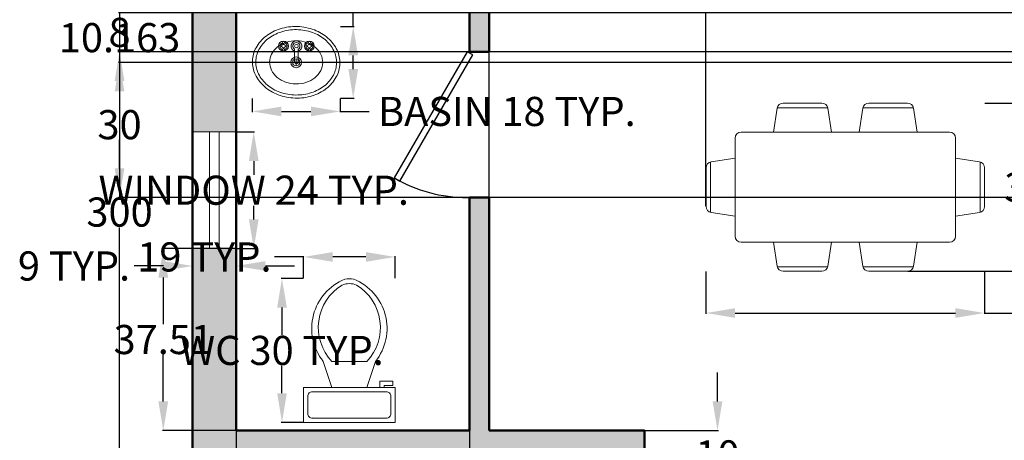
# Model space of a CAD drawing. Units: inches. Extents: x -11 to 341, y -300 to 41.
# Tile 2 of 5: x -11 to 192, y -178 to -91. Entities that reach past the tile are written whole.
import ezdxf

# ---------------------------------------------------------------- set-up
doc = ezdxf.new("R2010")
doc.units = ezdxf.units.IN
doc.header["$MEASUREMENT"] = 0
for name, color, linetype, lineweight in [('A-ANNO-DIMS', 2, 'Continuous', 18), ('A-DOOR', 3, 'Continuous', 25), ('A-FLOR-FIXT', 9, 'Continuous', 18), ('A-FURN', 8, 'Continuous', 18), ('A-GLAZ', 4, 'Continuous', 18), ('A-WALL', 7, 'Continuous', 50), ('A-WALL-PATT', 251, 'Continuous', 13)]:
    doc.layers.add(name, color=color, linetype=linetype, lineweight=lineweight)
doc.styles.get("Standard").update_dxf_attribs({"font": 'arial.ttf'})
doc.dimstyles.get("Standard").update_dxf_attribs({"dimtxt": 6, "dimasz": 6, "dimexe": 0.18, "dimexo": 0.0625, "dimgap": 0.09, "dimtad": 0, "dimtih": 1, "dimtoh": 1, "dimdec": 0, "dimzin": 0, "dimdsep": 46, "dimlunit": 4, "dimtxsty": 'Standard', "dimcen": 0.09, "dimadec": 0, "dimazin": 0, "dimtfac": 1, "dimtdec": 0, "dimtofl": 0, "dimtmove": 0, "dimatfit": 3, "dimfxl": 1, "dimtolj": 1, "dimtzin": 0, "dimarcsym": 0})

# ---------------------------------------------------------------- blocks, each defined once
blk = doc.blocks.new('*U15')
for p, q in [((0, 0), (0, 6)), ((40, 0), (40, 6))]:
    blk.add_line(p, q)
blk.add_lwpolyline([(0, 0), (34.64, -20), (35.52, -18.48), (0.87, 1.52)], close=True)
blk.add_arc((0, 0), 40, 330, 0)
blk = doc.blocks.new('Toilet - top')
for p, q in [((9.5, -6), (9.5, -2)), ((-10, -8.5), (-8, -8.5)), ((-10, -9.5), (-10, -8.5)), ((-8, -8.5), (-8, -8)), ((-7, -8), (-7, -9.5)), ((-4, -8), (-6, -14)), ((4, -8), (6, -14)), ((-7, -9.5), (-10, -9.5)), ((4, -14), (-4, -14))]:
    blk.add_line(p, q)
blk.add_lwpolyline([(10.5, -8), (10.5, 0), (-10.5, 0), (-10.5, -8)], close=True)
for points in [[(-9.5, -2), (-9.5, -6)], [(8.5, -1), (-8.5, -1)], [(-8.5, -7), (8.5, -7)]]:
    blk.add_lwpolyline(points)
for centre, radius, start, end in [((-8.62, -1.88), 0.884, 81.8699, 188.1301), ((8.62, -1.88), 0.884, 351.8699, 98.1301), ((-8.62, -6.12), 0.884, 171.8699, 278.1301), ((8.62, -6.12), 0.884, 261.8699, 8.1301), ((3.52, -21.58), 12.17, 141.4691, 247.9714), ((4.2, -21.82), 11.33, 136.3677, 238.9468), ((-3.52, -21.58), 12.17, 292.0284, 38.5307), ((-4.2, -21.82), 11.33, 301.053, 43.6321), ((0, -27.88), 4, 245.7318, 294.2682), ((0, -29), 4, 254.8605, 285.1395)]:
    blk.add_arc(centre, radius, start, end)
blk = doc.blocks.new('Sink - Oval top')
for p, q in [((-1, 0), (1, 0)), ((0, 1), (0, -1))]:
    blk.add_line(p, q)
for points in [[(-12.23, 0.39, 0.117634), (-11.46, -3.36, 0.104469), (-8.88, -6.8, 0.090016), (-5.08, -9.07, 0.08192), (-0.32, -10.02, 0.08192), (4.49, -9.38, 0.090016), (8.42, -7.36, 0.104469), (11.22, -4.09, 0.117634), (12.23, -0.39, 0.117634), (11.46, 3.36, 0.104469), (8.88, 6.8, 0.090016), (5.08, 9.07, 0.08192), (0.32, 10.02, 0.08192), (-4.49, 9.38, 0.090016), (-8.42, 7.36, 0.104469), (-11.22, 4.09, 0.117634)], [(-11.29, 0.16, 0.118622), (-10.52, -3.25, 0.104678), (-8.07, -6.36, 0.089562), (-4.54, -8.37, 0.081185), (-0.13, -9.15, 0.081185), (4.3, -8.49, 0.089562), (7.89, -6.58, 0.104678), (10.42, -3.55, 0.118622), (11.29, -0.16, 0.118622), (10.52, 3.25, 0.104678), (8.07, 6.36, 0.089562), (4.54, 8.37, 0.081185), (0.13, 9.15, 0.081185), (-4.3, 8.49, 0.089562), (-7.89, 6.58, 0.104678), (-10.42, 3.55, 0.118622)], [(-7.42, 0.08, 0.118283), (-6.91, -2.17, 0.104607), (-5.29, -4.21, 0.089718), (-2.97, -5.53, 0.081436), (-0.07, -6.04, 0.081436), (2.84, -5.59, 0.089718), (5.2, -4.33, 0.104607), (6.86, -2.32, 0.118283), (7.42, -0.08, 0.118283), (6.91, 2.17, 0.104607), (5.29, 4.21, 0.089718), (2.97, 5.53, 0.081436), (0.07, 6.04, 0.081436), (-2.84, 5.59, 0.089718), (-5.2, 4.33, 0.104607), (-6.86, 2.32, 0.118283)]]:
    blk.add_lwpolyline(points, format="xyb", close=True)
for radius in [1.5, 1]:
    blk.add_circle((0, 0), radius)
blk = doc.blocks.new('Faucet - Bathroom top')
for p, q in [((-4.107, 0.125), (-4.375, 0.125)), ((-3.75, 0.4788), (-3.75, 0.75)), ((-3.5, 0.482), (-3.5, 0.75)), ((-3.1461, 0.125), (-2.875, 0.125)), ((3.143, 0.125), (2.875, 0.125)), ((3.5, 0.4788), (3.5, 0.75)), ((3.75, 0.482), (3.75, 0.75)), ((4.1039, 0.125), (4.375, 0.125)), ((-4.1039, -0.125), (-4.375, -0.125)), ((-3.75, -0.4821), (-3.75, -0.75)), ((-3.5, -0.4789), (-3.5, -0.75)), ((-3.143, -0.125), (-2.875, -0.125)), ((-0.5, -0.8639), (-0.5, -4.5)), ((0.5, -4.5), (0.5, -0.8631)), ((3.1461, -0.125), (2.875, -0.125)), ((3.5, -0.4821), (3.5, -0.75)), ((3.75, -0.4789), (3.75, -0.75)), ((4.107, -0.125), (4.375, -0.125))]:
    blk.add_line(p, q)
for centre, radius in [((-3.625, 0), 1.375), ((-4.625, 0), 0.2795), ((-3.625, 0), 0.5), ((-3.625, 1), 0.2795), ((-2.625, 0), 0.2795), ((0, 0), 0.5), ((3.625, 0), 1.375), ((2.625, 0), 0.2795), ((3.625, 0), 0.5), ((3.625, 1), 0.2795), ((4.625, 0), 0.2795), ((-3.625, -1), 0.2795), ((3.625, -1), 0.2795)]:
    blk.add_circle(centre, radius)
for centre, radius, start, end in [((-3.625, 0), 1, 105.2407, 164.2093), ((-3.625, 0), 1, 16.44125, 74.07887), ((0, 0), 1.5, 289.6514, 250.3603), ((0, 0), 1, 300.3431, 239.7554), ((3.625, 0), 1, 106.12, 164.0884), ((3.625, 0), 1, 16.23422, 73.90469), ((-3.625, 0), 1, 196.2342, 253.9047), ((-3.625, 0), 1, 286.12, 344.0884), ((3.625, 0), 1, 196.4413, 254.0789), ((3.625, 0), 1, 285.2407, 344.2093), ((0, -4.5), 0.5, 180, 0)]:
    blk.add_arc(centre, radius, start, end)
blk = doc.blocks.new('Dining Set - 36 x 72 in.')
for p, q in [((-22.26, 25.81), (-23.48, 18)), ((-22.23, 26), (-5.76, 26)), ((-20.29, 27.5), (-7.71, 27.5)), ((-4.52, 18), (-5.74, 25.81)), ((5.74, 25.81), (4.52, 18)), ((5.77, 26), (22.24, 26)), ((7.71, 27.5), (20.29, 27.5)), ((23.48, 18), (22.26, 25.81)), ((34, 18), (-34, 18)), ((-36, 16), (-36, -16)), ((36, -16), (36, 16)), ((-44, 8.23), (-44, -8.24)), ((-43.81, 8.26), (-36, 9.48)), ((43.81, 8.26), (36, 9.48)), ((44, 8.23), (44, -8.24)), ((-45.5, 6.29), (-45.5, -6.29)), ((45.5, 6.29), (45.5, -6.29)), ((-36, -9.48), (-43.81, -8.26)), ((36, -9.48), (43.81, -8.26)), ((-34, -18), (34, -18)), ((-22.26, -25.81), (-23.48, -18)), ((-4.52, -18), (-5.74, -25.81)), ((5.74, -25.81), (4.52, -18)), ((23.48, -18), (22.26, -25.81)), ((-22.23, -26), (-5.76, -26)), ((-20.29, -27.5), (-7.71, -27.5)), ((5.77, -26), (22.24, -26)), ((7.71, -27.5), (20.29, -27.5))]:
    blk.add_line(p, q)
for centre, start, end in [((-20.29, 25.5), 90, 171.1198), ((-7.71, 25.5), 8.881, 90), ((7.71, 25.5), 90, 171.1198), ((20.29, 25.5), 8.881, 90), ((-34, 16), 90, 180), ((34, 16), 0, 90), ((-43.5, 6.29), 98.8806, 180), ((43.5, 6.29), 0, 81.1194), ((-43.5, -6.29), 180, 261.1194), ((43.5, -6.29), 278.8806, 0), ((-34, -16), 180, 270), ((34, -16), 270, 0), ((-20.29, -25.5), 188.8802, 270), ((-7.71, -25.5), 270, 351.1191), ((7.71, -25.5), 188.8802, 270), ((20.29, -25.5), 270, 351.1191)]:
    blk.add_arc(centre, 2, start, end)
blk = doc.blocks.new('WIN-24IN')
for p, q in [((0, 24), (9, 24)), ((3.5, 0), (3.5, 24)), ((5.5, 0), (5.5, 24)), ((9, 0), (0, 0))]:
    blk.add_line(p, q)
blk = doc.blocks.new('*D21')
at = {"layer": 'A-ANNO-DIMS', "color": 0, "lineweight": -2, "transparency": 16777216}
for p, q in [((33.63, -114.1), (37.35, -114.1)), ((37.17, -120.1), (37.17, -122.9)), ((37.17, -132.1), (37.17, -129.29)), ((33.63, -138.1), (37.35, -138.1))]:
    blk.add_line(p, q, dxfattribs=at)
at = {"layer": 'A-ANNO-DIMS', "color": 0, "transparency": 16777216}
for points in [[(36.17, -120.1), (38.17, -120.1), (37.17, -114.1)], [(36.17, -132.1), (38.17, -132.1), (37.17, -138.1)]]:
    blk.add_solid(points, dxfattribs=at)
at = {"layer": 'Defpoints', "color": 0, "transparency": 16777216}
for p in [(33.57, -114.1), (33.57, -138.1), (37.17, -138.1)]:
    blk.add_point(p, dxfattribs=at)
at = {"layer": 'A-ANNO-DIMS', "color": 0, "transparency": 16777216, "insert": (37.17, -126.1), "char_height": 6, "attachment_point": 5}
blk.add_mtext('\\A1;WINDOW 24 TYP.', dxfattribs=at)
blk = doc.blocks.new('*D22')
at = {"layer": 'A-ANNO-DIMS', "color": 0, "lineweight": -2, "transparency": 16777216}
for p, q in [((24.57, -138.16), (24.57, -141.88)), ((33.57, -138.16), (33.57, -141.88)), ((18.57, -141.7), (12.57, -141.7)), ((39.57, -141.7), (45.57, -141.7))]:
    blk.add_line(p, q, dxfattribs=at)
at = {"layer": 'A-ANNO-DIMS', "color": 0, "transparency": 16777216}
for points in [[(18.57, -140.7), (18.57, -142.7), (24.57, -141.7)], [(39.57, -140.7), (39.57, -142.7), (33.57, -141.7)]]:
    blk.add_solid(points, dxfattribs=at)
at = {"layer": 'Defpoints', "color": 0, "transparency": 16777216}
for p in [(24.57, -138.1), (33.57, -138.1), (24.57, -141.7)]:
    blk.add_point(p, dxfattribs=at)
at = {"layer": 'A-ANNO-DIMS', "color": 0, "transparency": 16777216, "insert": (0.2, -141.7), "char_height": 6, "attachment_point": 5}
blk.add_mtext('\\A1;9 TYP.', dxfattribs=at)
blk = doc.blocks.new('*D29')
at = {"layer": 'A-ANNO-DIMS', "color": 0, "lineweight": -2, "transparency": 16777216}
for p, q in [((47.36, -144.28), (42.8, -144.28)), ((42.98, -150.28), (42.98, -155.9)), ((42.98, -167.9), (42.98, -162.29)), ((47.36, -173.9), (42.8, -173.9))]:
    blk.add_line(p, q, dxfattribs=at)
at = {"layer": 'A-ANNO-DIMS', "color": 0, "transparency": 16777216}
for points in [[(41.98, -150.28), (43.98, -150.28), (42.98, -144.28)], [(41.98, -167.9), (43.98, -167.9), (42.98, -173.9)]]:
    blk.add_solid(points, dxfattribs=at)
at = {"layer": 'Defpoints', "color": 0, "transparency": 16777216}
for p in [(47.43, -144.28), (42.98, -173.9), (47.43, -173.9)]:
    blk.add_point(p, dxfattribs=at)
at = {"layer": 'A-ANNO-DIMS', "color": 0, "transparency": 16777216, "insert": (42.98, -159.09), "char_height": 6, "attachment_point": 5}
blk.add_mtext('\\A1;WC 30 TYP.', dxfattribs=at)
blk = doc.blocks.new('*D30')
at = {"layer": 'A-ANNO-DIMS', "color": 0, "lineweight": -2, "transparency": 16777216}
for p, q in [((47.43, -144.22), (47.43, -139.66)), ((66.25, -144.22), (66.25, -139.66)), ((47.43, -139.84), (41.43, -139.84)), ((60.25, -139.84), (53.43, -139.84))]:
    blk.add_line(p, q, dxfattribs=at)
at = {"layer": 'A-ANNO-DIMS', "color": 0, "transparency": 16777216}
for points in [[(53.43, -138.84), (53.43, -140.84), (47.43, -139.84)], [(60.25, -138.84), (60.25, -140.84), (66.25, -139.84)]]:
    blk.add_solid(points, dxfattribs=at)
at = {"layer": 'Defpoints', "color": 0, "transparency": 16777216}
for p in [(47.43, -139.84), (47.43, -144.28), (66.25, -144.28)]:
    blk.add_point(p, dxfattribs=at)
at = {"layer": 'A-ANNO-DIMS', "color": 0, "transparency": 16777216, "insert": (27.02, -139.84), "char_height": 6, "attachment_point": 5}
blk.add_mtext('\\A1;19 TYP.', dxfattribs=at)
blk = doc.blocks.new('*D31')
at = {"layer": 'A-ANNO-DIMS', "color": 0, "lineweight": -2, "transparency": 16777216}
for p, q in [((36.87, -107.23), (36.87, -110.06)), ((54.93, -107.23), (54.93, -110.06)), ((42.87, -109.88), (48.93, -109.88)), ((54.93, -109.88), (60.93, -109.88))]:
    blk.add_line(p, q, dxfattribs=at)
at = {"layer": 'A-ANNO-DIMS', "color": 0, "transparency": 16777216}
for points in [[(42.87, -108.88), (42.87, -110.88), (36.87, -109.88)], [(48.93, -108.88), (48.93, -110.88), (54.93, -109.88)]]:
    blk.add_solid(points, dxfattribs=at)
at = {"layer": 'Defpoints', "color": 0, "transparency": 16777216}
for p in [(36.87, -107.17), (54.93, -107.17), (54.93, -109.88)]:
    blk.add_point(p, dxfattribs=at)
at = {"layer": 'A-ANNO-DIMS', "color": 0, "transparency": 16777216, "insert": (89.23, -109.88), "char_height": 6, "attachment_point": 5}
blk.add_mtext('\\A1;BASIN 18 TYP.', dxfattribs=at)
blk = doc.blocks.new('*D32')
at = {"layer": 'A-ANNO-DIMS', "color": 0, "lineweight": -2, "transparency": 16777216}
for p, q in [((57.63, -92.36), (57.63, -86.36)), ((57.63, -86.36), (63.63, -86.36)), ((54.99, -92.36), (57.81, -92.36)), ((57.63, -101.17), (57.63, -98.36)), ((54.99, -107.17), (57.81, -107.17))]:
    blk.add_line(p, q, dxfattribs=at)
at = {"layer": 'A-ANNO-DIMS', "color": 0, "transparency": 16777216}
for points in [[(56.63, -98.36), (58.63, -98.36), (57.63, -92.36)], [(56.63, -101.17), (58.63, -101.17), (57.63, -107.17)]]:
    blk.add_solid(points, dxfattribs=at)
at = {"layer": 'Defpoints', "color": 0, "transparency": 16777216}
for p in [(54.93, -92.36), (57.63, -92.36), (54.93, -107.17)]:
    blk.add_point(p, dxfattribs=at)
at = {"layer": 'A-ANNO-DIMS', "color": 0, "transparency": 16777216, "insert": (78.05, -86.36), "char_height": 6, "attachment_point": 5}
blk.add_mtext('\\A1;15 TYP.', dxfattribs=at)
blk = doc.blocks.new('*D43')
at = {"layer": 'A-ANNO-DIMS', "color": 0, "lineweight": -2, "transparency": 16777216}
for p, q in [((130.2, -142.86), (130.2, -151.57)), ((187.51, -142.86), (187.51, -151.57)), ((136.2, -151.39), (181.51, -151.39)), ((187.51, -151.39), (193.51, -151.39))]:
    blk.add_line(p, q, dxfattribs=at)
at = {"layer": 'A-ANNO-DIMS', "color": 0, "transparency": 16777216}
for points in [[(136.2, -150.39), (136.2, -152.39), (130.2, -151.39)], [(181.51, -150.39), (181.51, -152.39), (187.51, -151.39)]]:
    blk.add_solid(points, dxfattribs=at)
at = {"layer": 'Defpoints', "color": 0, "transparency": 16777216}
for p in [(130.2, -142.8), (187.51, -142.8), (187.51, -151.39)]:
    blk.add_point(p, dxfattribs=at)
at = {"layer": 'A-ANNO-DIMS', "color": 0, "transparency": 16777216, "insert": (222.9, -151.39), "char_height": 6, "attachment_point": 5}
blk.add_mtext('\\A1;DINING SET 57', dxfattribs=at)
blk = doc.blocks.new('*D44')
at = {"layer": 'A-ANNO-DIMS', "color": 0, "lineweight": -2, "transparency": 16777216}
for p, q in [((187.57, -108.16), (196.29, -108.16)), ((196.11, -114.16), (196.11, -122.32)), ((196.11, -136.8), (196.11, -128.63)), ((187.57, -142.8), (196.29, -142.8))]:
    blk.add_line(p, q, dxfattribs=at)
at = {"layer": 'A-ANNO-DIMS', "color": 0, "transparency": 16777216}
for points in [[(195.11, -114.16), (197.11, -114.16), (196.11, -108.16)], [(195.11, -136.8), (197.11, -136.8), (196.11, -142.8)]]:
    blk.add_solid(points, dxfattribs=at)
at = {"layer": 'Defpoints', "color": 0, "transparency": 16777216}
for p in [(187.51, -108.16), (196.11, -108.16), (187.51, -142.8)]:
    blk.add_point(p, dxfattribs=at)
at = {"layer": 'A-ANNO-DIMS', "color": 0, "transparency": 16777216, "insert": (196.11, -125.48), "char_height": 6, "attachment_point": 5}
blk.add_mtext('\\A1;35', dxfattribs=at)
blk = doc.blocks.new('*D46')
at = {"layer": 'A-ANNO-DIMS', "color": 0, "lineweight": -2, "transparency": 16777216}
for p, q in [((24.5, 19.4), (9.38, 19.4)), ((9.56, 13.4), (9.56, -127.45)), ((9.56, -274.6), (9.56, -133.76)), ((24.5, -280.6), (9.38, -280.6))]:
    blk.add_line(p, q, dxfattribs=at)
at = {"layer": 'A-ANNO-DIMS', "color": 0, "transparency": 16777216}
for points in [[(8.56, 13.4), (10.56, 13.4), (9.56, 19.4)], [(8.56, -274.6), (10.56, -274.6), (9.56, -280.6)]]:
    blk.add_solid(points, dxfattribs=at)
at = {"layer": 'Defpoints', "color": 0, "transparency": 16777216}
for p in [(9.56, 19.4), (24.57, 19.4), (24.57, -280.6)]:
    blk.add_point(p, dxfattribs=at)
at = {"layer": 'A-ANNO-DIMS', "color": 0, "transparency": 16777216, "insert": (9.56, -130.6), "char_height": 6, "attachment_point": 5}
blk.add_mtext('\\A1;300', dxfattribs=at)
blk = doc.blocks.new('*D61')
at = {"layer": 'A-ANNO-DIMS', "color": 0, "lineweight": -2, "transparency": 16777216}
for p, q in [((33.57, -175.67), (33.57, -190.79)), ((81.57, -175.67), (81.57, -190.79)), ((39.57, -190.61), (53.05, -190.61)), ((75.57, -190.61), (62.08, -190.61))]:
    blk.add_line(p, q, dxfattribs=at)
at = {"layer": 'A-ANNO-DIMS', "color": 0, "transparency": 16777216}
for points in [[(39.57, -189.61), (39.57, -191.61), (33.57, -190.61)], [(75.57, -189.61), (75.57, -191.61), (81.57, -190.61)]]:
    blk.add_solid(points, dxfattribs=at)
at = {"layer": 'Defpoints', "color": 0, "transparency": 16777216}
for p in [(33.57, -175.6), (81.57, -175.6), (33.57, -190.61)]:
    blk.add_point(p, dxfattribs=at)
at = {"layer": 'A-ANNO-DIMS', "color": 0, "transparency": 16777216, "insert": (57.57, -190.61), "char_height": 6, "attachment_point": 5}
blk.add_mtext('\\A1;48', dxfattribs=at)
blk = doc.blocks.new('*D62')
at = {"layer": 'A-ANNO-DIMS', "color": 0, "lineweight": -2, "transparency": 16777216}
for p, q in [((85.57, -175.54), (85.57, 34.58)), ((227.57, -175.54), (227.57, 34.58)), ((91.57, 34.4), (150.16, 34.4)), ((221.57, 34.4), (162.97, 34.4))]:
    blk.add_line(p, q, dxfattribs=at)
at = {"layer": 'A-ANNO-DIMS', "color": 0, "transparency": 16777216}
for points in [[(91.57, 35.4), (91.57, 33.4), (85.57, 34.4)], [(221.57, 35.4), (221.57, 33.4), (227.57, 34.4)]]:
    blk.add_solid(points, dxfattribs=at)
at = {"layer": 'Defpoints', "color": 0, "transparency": 16777216}
for p in [(227.57, 34.4), (85.57, -175.6), (227.57, -175.6)]:
    blk.add_point(p, dxfattribs=at)
at = {"layer": 'A-ANNO-DIMS', "color": 0, "transparency": 16777216, "insert": (156.57, 34.4), "char_height": 6, "attachment_point": 5}
blk.add_mtext('\\A1;142', dxfattribs=at)
blk = doc.blocks.new('*D64')
at = {"layer": 'A-ANNO-DIMS', "color": 0, "lineweight": -2, "transparency": 16777216}
for p, q in [((33.5, -138.1), (18.38, -138.1)), ((18.56, -144.1), (18.56, -153.69)), ((18.56, -169.6), (18.56, -160.01)), ((33.5, -175.6), (18.38, -175.6))]:
    blk.add_line(p, q, dxfattribs=at)
at = {"layer": 'A-ANNO-DIMS', "color": 0, "transparency": 16777216}
for points in [[(17.56, -144.1), (19.56, -144.1), (18.56, -138.1)], [(17.56, -169.6), (19.56, -169.6), (18.56, -175.6)]]:
    blk.add_solid(points, dxfattribs=at)
at = {"layer": 'Defpoints', "color": 0, "transparency": 16777216}
for p in [(18.56, -138.1), (33.57, -138.1), (33.57, -175.6)]:
    blk.add_point(p, dxfattribs=at)
at = {"layer": 'A-ANNO-DIMS', "color": 0, "transparency": 16777216, "insert": (18.56, -156.85), "char_height": 6, "attachment_point": 5}
blk.add_mtext('\\A1;37.51', dxfattribs=at)
blk = doc.blocks.new('*D66')
at = {"layer": 'A-ANNO-DIMS', "color": 0, "lineweight": -2, "transparency": 16777216}
for p, q in [((9.563121, -83.603265), (9.563121, -77.603265)), ((231.502621, -89.603265), (9.383121, -89.603265)), ((231.502621, -97.603265), (9.383121, -97.603265)), ((9.563121, -103.603265), (9.563121, -109.603265))]:
    blk.add_line(p, q, dxfattribs=at)
at = {"layer": 'A-ANNO-DIMS', "color": 0, "transparency": 16777216}
for points in [[(8.563121, -83.603265), (10.563121, -83.603265), (9.563121, -89.603265)], [(8.563121, -103.603265), (10.563121, -103.603265), (9.563121, -97.603265)]]:
    blk.add_solid(points, dxfattribs=at)
at = {"layer": 'Defpoints', "color": 0, "transparency": 16777216}
for p in [(231.565121, -89.603265), (9.563121, -97.603265), (231.565121, -97.603265)]:
    blk.add_point(p, dxfattribs=at)
at = {"layer": 'A-ANNO-DIMS', "color": 0, "transparency": 16777216, "insert": (9.563121, -93.603265), "char_height": 6, "attachment_point": 5}
blk.add_mtext('\\A1;8', dxfattribs=at)
blk = doc.blocks.new('*D67')
at = {"layer": 'A-ANNO-DIMS', "color": 0, "lineweight": -2, "transparency": 16777216}
for p, q in [((231.5, -97.6), (9.38, -97.6)), ((9.56, -103.6), (9.56, -109.45)), ((9.56, -121.6), (9.56, -115.76)), ((231.5, -127.6), (9.38, -127.6))]:
    blk.add_line(p, q, dxfattribs=at)
at = {"layer": 'A-ANNO-DIMS', "color": 0, "transparency": 16777216}
for points in [[(8.56, -103.6), (10.56, -103.6), (9.56, -97.6)], [(8.56, -121.6), (10.56, -121.6), (9.56, -127.6)]]:
    blk.add_solid(points, dxfattribs=at)
at = {"layer": 'Defpoints', "color": 0, "transparency": 16777216}
for p in [(9.56, -97.6), (231.57, -97.6), (231.57, -127.6)]:
    blk.add_point(p, dxfattribs=at)
at = {"layer": 'A-ANNO-DIMS', "color": 0, "transparency": 16777216, "insert": (9.56, -112.6), "char_height": 6, "attachment_point": 5}
blk.add_mtext('\\A1;30', dxfattribs=at)
blk = doc.blocks.new('*D70')
at = {"layer": 'A-ANNO-DIMS', "color": 0, "lineweight": -2, "transparency": 16777216}
for p, q in [((132.567121, -169.603265), (132.567121, -163.603265)), ((117.627621, -175.603265), (132.747121, -175.603265)), ((117.627621, -185.603265), (132.747121, -185.603265)), ((132.567121, -191.603265), (132.567121, -197.603265))]:
    blk.add_line(p, q, dxfattribs=at)
at = {"layer": 'A-ANNO-DIMS', "color": 0, "transparency": 16777216}
for points in [[(131.567121, -169.603265), (133.567121, -169.603265), (132.567121, -175.603265)], [(131.567121, -191.603265), (133.567121, -191.603265), (132.567121, -185.603265)]]:
    blk.add_solid(points, dxfattribs=at)
at = {"layer": 'Defpoints', "color": 0, "transparency": 16777216}
for p in [(117.565121, -175.603265), (117.565121, -185.603265), (132.567121, -185.603265)]:
    blk.add_point(p, dxfattribs=at)
at = {"layer": 'A-ANNO-DIMS', "color": 0, "transparency": 16777216, "insert": (132.567121, -180.603265), "char_height": 6, "attachment_point": 5}
blk.add_mtext('\\A1;10', dxfattribs=at)
blk = doc.blocks.new('*D84')
at = {"layer": 'A-ANNO-DIMS', "color": 0, "lineweight": -2, "transparency": 16777216}
for p, q in [((9.56, -83.6), (9.56, -77.6)), ((279.5, -89.6), (9.38, -89.6)), ((267.79, -99.77), (9.38, -99.77)), ((9.56, -105.77), (9.56, -111.77))]:
    blk.add_line(p, q, dxfattribs=at)
at = {"layer": 'A-ANNO-DIMS', "color": 0, "transparency": 16777216}
for points in [[(8.56, -83.6), (10.56, -83.6), (9.56, -89.6)], [(8.56, -105.77), (10.56, -105.77), (9.56, -99.77)]]:
    blk.add_solid(points, dxfattribs=at)
at = {"layer": 'Defpoints', "color": 0, "transparency": 16777216}
for p in [(9.56, -89.6), (279.57, -89.6), (267.86, -99.77)]:
    blk.add_point(p, dxfattribs=at)
at = {"layer": 'A-ANNO-DIMS', "color": 0, "transparency": 16777216, "insert": (9.56, -94.68), "char_height": 6, "attachment_point": 5}
blk.add_mtext('\\A1;10.163', dxfattribs=at)
blk = doc.blocks.new('*D85')
at = {"layer": 'A-ANNO-DIMS', "color": 0, "lineweight": -2, "transparency": 16777216}
for p, q in [((85.57, -127.54), (85.57, 34.58)), ((130.2, -129.38), (130.2, 34.58)), ((91.57, 34.4), (97.56, 34.4)), ((124.2, 34.4), (118.21, 34.4))]:
    blk.add_line(p, q, dxfattribs=at)
at = {"layer": 'A-ANNO-DIMS', "color": 0, "transparency": 16777216}
for points in [[(91.57, 35.4), (91.57, 33.4), (85.57, 34.4)], [(124.2, 35.4), (124.2, 33.4), (130.2, 34.4)]]:
    blk.add_solid(points, dxfattribs=at)
at = {"layer": 'Defpoints', "color": 0, "transparency": 16777216}
for p in [(130.2, 34.4), (85.57, -127.6), (130.2, -129.44)]:
    blk.add_point(p, dxfattribs=at)
at = {"layer": 'A-ANNO-DIMS', "color": 0, "transparency": 16777216, "insert": (107.88, 34.4), "char_height": 6, "attachment_point": 5}
blk.add_mtext('\\A1;44.64', dxfattribs=at)
blk = doc.blocks.new('*D86')
at = {"layer": 'A-ANNO-DIMS', "color": 0, "lineweight": -2, "transparency": 16777216}
for p, q in [((171.7, -142.8), (303.75, -142.8)), ((303.57, -148.8), (303.57, -156.04)), ((303.57, -169.6), (303.57, -162.36)), ((227.63, -175.6), (303.75, -175.6))]:
    blk.add_line(p, q, dxfattribs=at)
at = {"layer": 'A-ANNO-DIMS', "color": 0, "transparency": 16777216}
for points in [[(302.57, -148.8), (304.57, -148.8), (303.57, -142.8)], [(302.57, -169.6), (304.57, -169.6), (303.57, -175.6)]]:
    blk.add_solid(points, dxfattribs=at)
at = {"layer": 'Defpoints', "color": 0, "transparency": 16777216}
for p in [(171.63, -142.8), (303.57, -142.8), (227.57, -175.6)]:
    blk.add_point(p, dxfattribs=at)
at = {"layer": 'A-ANNO-DIMS', "color": 0, "transparency": 16777216, "insert": (303.57, -159.2), "char_height": 6, "attachment_point": 5}
blk.add_mtext('\\A1;32.806', dxfattribs=at)

msp = doc.modelspace()

# ---------------------------------------------------------------- hatches: boundary and pattern name
at = {"layer": 'A-WALL-PATT'}
h = msp.add_hatch(color=256, dxfattribs=at)
h.dxf.hatch_style = 1
h.paths.add_polyline_path([(33.5651, 10.3967), (49.4488, 10.3967), (49.4488, 19.3967), (24.5651, 19.3967), (24.5651, -114.096), (33.5651, -114.096), (33.5651, -89.6033), (81.5651, -89.6033), (81.5651, -97.6033), (85.5651, -97.6033), (85.5651, -89.6033), (89.5651, -89.6033), (89.5651, -86.0033), (89.5651, -85.6033), (33.5651, -85.6033)])
h = msp.add_hatch(color=256, dxfattribs=at)
h.dxf.hatch_style = 1
h.paths.add_polyline_path([(24.5651, -280.6033), (49.1398, -280.6033), (49.1398, -271.6033), (33.5651, -271.6033), (33.5651, -179.6033), (113.5651, -179.6033), (113.5651, -185.6033), (117.5651, -185.6033), (117.5651, -175.6033), (85.5651, -175.6033), (85.5651, -127.6033), (81.5651, -127.6033), (81.5651, -175.6033), (33.5651, -175.6033), (33.5651, -138.096), (24.5651, -138.096)])

# ---------------------------------------------------------------- linework, layer by layer
at = {"layer": 'A-WALL'}
for p, q in [((33.5651, -175.6033), (33.5651, -89.6033)), ((81.5651, -97.6033), (81.5651, -89.6033)), ((85.5651, -97.6033), (85.5651, -89.6033)), ((81.5651, -97.6033), (85.5651, -97.6033)), ((81.5651, -175.6033), (81.5651, -127.6033)), ((81.5651, -127.6033), (85.5651, -127.6033)), ((85.5651, -175.6033), (85.5651, -127.6033)), ((81.5651, -175.6033), (33.5651, -175.6033)), ((117.5651, -175.6033), (85.5651, -175.6033)), ((117.5651, -185.6033), (117.5651, -175.6033))]:
    msp.add_line(p, q, dxfattribs=at)
msp.add_lwpolyline([(129.5651, -280.6033), (24.5651, -280.6033), (24.5651, 19.3967), (288.5651, 19.3967), (288.5651, -280.6033), (165.5651, -280.6033)], dxfattribs=at)

# ---------------------------------------------------------------- block references
at = {"layer": 'A-DOOR', "xscale": 0.75, "yscale": 0.75, "zscale": 0.75, "rotation": 270}
msp.add_blockref('*U15', (81.0651, -97.6033), dxfattribs=at)
at = {"layer": 'A-FLOR-FIXT', "xscale": 0.7353737338940184, "yscale": 0.7353737338940184, "zscale": 0.7353737338940184}
for name, p in [('Sink - Oval top', (45.8994, -99.7667)), ('Faucet - Bathroom top', (45.949, -96.4304))]:
    msp.add_blockref(name, p, dxfattribs=at)
at = {"layer": 'A-FLOR-FIXT', "xscale": 0.896325363236769, "yscale": 0.896325363236769, "zscale": 0.896325363236769, "rotation": 180}
msp.add_blockref('Toilet - top', (56.8371, -173.9025), dxfattribs=at)
at = {"layer": 'A-FURN', "xscale": 0.6297572799486942, "yscale": 0.6297572799486942, "zscale": 0.6297572799486942}
msp.add_blockref('Dining Set - 36 x 72 in.', (158.858, -125.4794), dxfattribs=at)
at = {"layer": 'A-GLAZ', "rotation": 180}
msp.add_blockref('WIN-24IN', (33.5652, -114.0963), dxfattribs=at)

# ---------------------------------------------------------------- dimensions: what is measured, and where the dimension line sits
at = {"layer": 'A-ANNO-DIMS'}
for base, p1, p2, override, picture, middle in [((227.5651, 34.3987), (85.5651, -175.6033), (227.5651, -175.6033), {"dimdec": 0, "dimlfac": 1, "dimrnd": 0, "dimzin": 0, "dimdsep": 46, "dimlunit": 2}, '*D62', (156.5651, 34.3987)), ((130.204, 34.3987), (85.5651, -127.6033), (130.204, -129.4394), {"dimdec": 2, "dimlfac": 1, "dimrnd": 0, "dimzin": 0, "dimdsep": 46, "dimlunit": 2}, '*D85', (107.8846, 34.3987))]:
    dim = msp.add_linear_dim(base=base, p1=p1, p2=p2, dimstyle='Standard', override=override, dxfattribs=at)
    dim.commit()
    dim.dimension.update_dxf_attribs({"geometry": picture, "text_midpoint": middle})
for base, p1, p2, angle, override, picture, middle in [((9.5631, 19.3967), (24.5651, -280.6033), (24.5651, 19.3967), 90, {"dimdec": 0, "dimlfac": 1, "dimrnd": 0, "dimzin": 0, "dimdsep": 46, "dimlunit": 2}, '*D46', (9.5631, -130.6033)), ((9.5631, -89.6033), (267.8569, -99.7667), (279.5651, -89.6033), 90, {"dimdec": 3, "dimlfac": 1, "dimrnd": 0, "dimzin": 0, "dimdsep": 46, "dimlunit": 2}, '*D84', (9.5631, -94.685)), ((9.5631, -97.6033), (231.5651, -89.6033), (231.5651, -97.6033), 90, {"dimdec": 0, "dimlfac": 1, "dimrnd": 0, "dimzin": 0, "dimdsep": 46, "dimlunit": 2}, '*D66', (9.5631, -93.6033)), ((9.5631, -97.6033), (231.5651, -127.6033), (231.5651, -97.6033), 90, {"dimdec": 0, "dimlfac": 1, "dimrnd": 0, "dimzin": 0, "dimdsep": 46, "dimlunit": 2}, '*D67', (9.5631, -112.6033)), ((196.1081, -108.161), (187.5119, -142.7977), (187.5119, -108.161), 90, {"dimdec": 0, "dimlfac": 1, "dimrnd": 0, "dimzin": 0, "dimdsep": 46, "dimlunit": 2}, '*D44', (196.1081, -125.4794)), ((18.5631, -138.096), (33.5651, -175.6033), (33.5651, -138.096), 90, {"dimdec": 2, "dimlfac": 1, "dimrnd": 0, "dimzin": 0, "dimdsep": 46, "dimlunit": 2}, '*D64', (18.5631, -156.8496)), ((303.5671, -142.7977), (227.5651, -175.6033), (171.6347, -142.7977), 90, {"dimdec": 3, "dimlfac": 1, "dimrnd": 0, "dimzin": 0, "dimdsep": 46, "dimlunit": 2}, '*D86', (303.5671, -159.2005)), ((132.5671, -185.6033), (117.5651, -175.6033), (117.5651, -185.6033), 270, {"dimdec": 0, "dimlfac": 1, "dimrnd": 0, "dimzin": 0, "dimdsep": 46, "dimlunit": 2}, '*D70', (132.5671, -180.6033)), ((33.5651, -190.6053), (81.5651, -175.6033), (33.5651, -175.6033), 180, {"dimdec": 0, "dimlfac": 1, "dimrnd": 0, "dimzin": 0, "dimdsep": 46, "dimlunit": 2}, '*D61', (57.5651, -190.6053))]:
    dim = msp.add_linear_dim(base=base, p1=p1, p2=p2, angle=angle, dimstyle='Standard', override=override, dxfattribs=at)
    dim.commit()
    dim.dimension.update_dxf_attribs({"geometry": picture, "text_midpoint": middle})
for base, p1, p2, angle, text, picture, middle in [((57.6345, -92.3627), (54.9264, -107.1706), (54.9264, -92.3627), 90, '<> TYP.', '*D32', (78.0451, -86.3627)), ((37.1651, -138.096), (33.5651, -114.096), (33.5651, -138.096), 270, 'WINDOW <> TYP.', '*D21', (37.1651, -126.096)), ((47.4256, -139.8392), (66.2485, -144.2823), (47.4256, -144.2823), 180, '<> TYP.', '*D30', (27.015, -139.8392)), ((24.5651, -141.696), (33.5651, -138.096), (24.5651, -138.096), 180, '<> TYP.', '*D22', (0.203, -141.696)), ((42.9826, -173.9025), (47.4256, -144.2823), (47.4256, -173.9025), 270, 'WC <> TYP.', '*D29', (42.9826, -159.0924))]:
    dim = msp.add_linear_dim(base=base, p1=p1, p2=p2, angle=angle, text=text, dimstyle='Standard', override={"dimdec": 0, "dimlfac": 1, "dimrnd": 0, "dimzin": 0, "dimdsep": 46, "dimlunit": 2}, dxfattribs=at)
    dim.commit()
    dim.dimension.update_dxf_attribs({"geometry": picture, "text_midpoint": middle})
for base, p1, p2, text, picture, middle in [((54.9264, -109.8787), (36.8723, -107.1706), (54.9264, -107.1706), 'BASIN <> TYP.', '*D31', (89.2279, -109.8787)), ((187.5119, -151.3939), (130.204, -142.7977), (187.5119, -142.7977), 'DINING SET <>', '*D43', (222.898, -151.3939))]:
    dim = msp.add_linear_dim(base=base, p1=p1, p2=p2, text=text, dimstyle='Standard', override={"dimdec": 0, "dimlfac": 1, "dimrnd": 0, "dimzin": 0, "dimdsep": 46, "dimlunit": 2}, dxfattribs=at)
    dim.commit()
    dim.dimension.update_dxf_attribs({"geometry": picture, "text_midpoint": middle})

doc.saveas('drawing.dxf')
